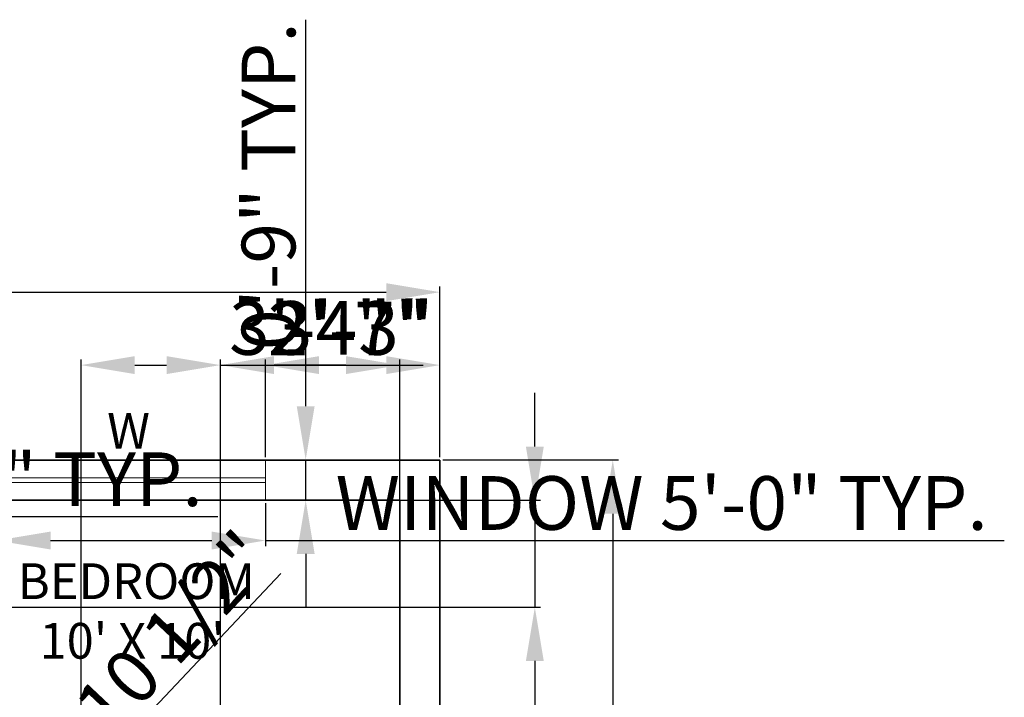
# Model space of a CAD drawing. Units: inches. Extents: x 2122 to 2726, y 1923 to 2370.
# Tile 6 of 6: x 2506 to 2726, y 2218 to 2370. Entities that reach past the tile are written whole.
import ezdxf

# ---------------------------------------------------------------- set-up
doc = ezdxf.new("R2010")
doc.units = ezdxf.units.IN
for name, color, linetype, lineweight in [('A-ANNO-DIMS', 2, 'Continuous', 18), ('A-ANNO-TEXT', 7, 'Continuous', 18), ('A-AREA-IDEN', 7, 'Continuous', 25), ('A-GLAZ', 4, 'Continuous', 18), ('A-WALL', 7, 'Continuous', 35)]:
    doc.layers.add(name, color=color, linetype=linetype, lineweight=lineweight)
doc.styles.get("Standard").update_dxf_attribs({"font": 'arial.ttf'})
doc.dimstyles.new('ISO-25', dxfattribs={"dimtxt": 12, "dimasz": 12, "dimexe": 1.25, "dimexo": 0.625, "dimtad": 1, "dimlunit": 3, "dimtxsty": 'Standard', "dimcen": 2.5, "dimadec": 0, "dimazin": 0, "dimtfac": 1, "dimtmove": 0, "dimatfit": 3, "dimfxl": 1, "dimarcsym": 0})

# ---------------------------------------------------------------- blocks, each defined once
blk = doc.blocks.new('*D9')
at = {"layer": 'A-ANNO-DIMS', "color": 0, "lineweight": -2, "transparency": 16777216}
for p, q in [((2600.63, 2271.24), (2639.88, 2271.24)), ((2638.63, 2259.24), (2638.63, 1984.74)), ((2600.63, 1972.74), (2639.88, 1972.74))]:
    blk.add_line(p, q, dxfattribs=at)
at = {"layer": 'A-ANNO-DIMS', "color": 0, "transparency": 16777216}
for points in [[(2636.63, 2259.24), (2640.63, 2259.24), (2638.63, 2271.24)], [(2636.63, 1984.74), (2640.63, 1984.74), (2638.63, 1972.74)]]:
    blk.add_solid(points, dxfattribs=at)
at = {"layer": 'Defpoints', "color": 0, "transparency": 16777216}
for p in [(2600.01, 2271.24), (2600.01, 1972.74), (2638.63, 1972.74)]:
    blk.add_point(p, dxfattribs=at)
at = {"layer": 'A-ANNO-DIMS', "color": 0, "transparency": 16777216, "insert": (2631.88, 2121.99), "char_height": 12, "attachment_point": 5, "rotation": 90}
blk.add_mtext("25'", dxfattribs=at)
blk = doc.blocks.new('*D10')
at = {"layer": 'A-ANNO-DIMS', "color": 0, "lineweight": -2, "transparency": 16777216}
for p, q in [((2232.51, 2271.86), (2232.51, 2309.99)), ((2244.51, 2308.74), (2588.01, 2308.74)), ((2600.01, 2271.86), (2600.01, 2309.99))]:
    blk.add_line(p, q, dxfattribs=at)
at = {"layer": 'A-ANNO-DIMS', "color": 0, "transparency": 16777216}
for points in [[(2244.51, 2310.74), (2244.51, 2306.74), (2232.51, 2308.74)], [(2588.01, 2310.74), (2588.01, 2306.74), (2600.01, 2308.74)]]:
    blk.add_solid(points, dxfattribs=at)
at = {"layer": 'Defpoints', "color": 0, "transparency": 16777216}
for p in [(2600.01, 2308.74), (2232.51, 2271.24), (2600.01, 2271.24)]:
    blk.add_point(p, dxfattribs=at)
at = {"layer": 'A-ANNO-DIMS', "color": 0, "transparency": 16777216, "insert": (2416.26, 2315.49), "char_height": 12, "attachment_point": 5}
blk.add_mtext("31'", dxfattribs=at)
blk = doc.blocks.new('WIN-60IN')
for p, q in [((0, 0), (0, 9)), ((60, 0), (60, 9)), ((0, 5), (60, 5)), ((0, 4), (60, 4))]:
    blk.add_line(p, q)
blk = doc.blocks.new('*D16')
at = {"layer": 'A-ANNO-DIMS', "color": 0, "lineweight": -2, "transparency": 16777216}
for p, q in [((2501.01, 2261.61), (2501.01, 2251.99)), ((2561.01, 2261.61), (2561.01, 2251.99)), ((2513.01, 2253.24), (2549.01, 2253.24)), ((2561.01, 2253.24), (2726.11, 2253.24))]:
    blk.add_line(p, q, dxfattribs=at)
at = {"layer": 'A-ANNO-DIMS', "color": 0, "transparency": 16777216}
for points in [[(2513.01, 2255.24), (2513.01, 2251.24), (2501.01, 2253.24)], [(2549.01, 2255.24), (2549.01, 2251.24), (2561.01, 2253.24)]]:
    blk.add_solid(points, dxfattribs=at)
at = {"layer": 'Defpoints', "color": 0, "transparency": 16777216}
for p in [(2501.01, 2262.24), (2561.01, 2262.24), (2561.01, 2253.24)]:
    blk.add_point(p, dxfattribs=at)
at = {"layer": 'A-ANNO-DIMS', "color": 0, "transparency": 16777216, "insert": (2649.56, 2260.07), "char_height": 12, "attachment_point": 5}
blk.add_mtext('WINDOW 5\'-0" TYP.', dxfattribs=at)
blk = doc.blocks.new('*D17')
at = {"layer": 'A-ANNO-DIMS', "color": 0, "lineweight": -2, "transparency": 16777216}
for p, q in [((2570.01, 2283.24), (2570.01, 2369.63)), ((2561.63, 2271.24), (2571.26, 2271.24)), ((2570.01, 2262.24), (2570.01, 2271.24)), ((2561.63, 2262.24), (2571.26, 2262.24)), ((2570.01, 2250.24), (2570.01, 2238.24))]:
    blk.add_line(p, q, dxfattribs=at)
at = {"layer": 'A-ANNO-DIMS', "color": 0, "transparency": 16777216}
for points in [[(2568.01, 2283.24), (2572.01, 2283.24), (2570.01, 2271.24)], [(2568.01, 2250.24), (2572.01, 2250.24), (2570.01, 2262.24)]]:
    blk.add_solid(points, dxfattribs=at)
at = {"layer": 'Defpoints', "color": 0, "transparency": 16777216}
for p in [(2561.01, 2271.24), (2570.01, 2271.24), (2561.01, 2262.24)]:
    blk.add_point(p, dxfattribs=at)
at = {"layer": 'A-ANNO-DIMS', "color": 0, "transparency": 16777216, "insert": (2563.26, 2332.43), "char_height": 12, "attachment_point": 5, "rotation": 90}
blk.add_mtext('0\'-9" TYP.', dxfattribs=at)
blk = doc.blocks.new('*D20')
at = {"layer": 'A-ANNO-DIMS', "color": 0, "lineweight": -2, "transparency": 16777216}
for p, q in [((2378.01, 2261.61), (2378.01, 2257.39)), ((2402.01, 2261.61), (2402.01, 2257.39)), ((2366.01, 2258.64), (2354.01, 2258.64)), ((2378.01, 2258.64), (2402.01, 2258.64)), ((2414.01, 2258.64), (2550.39, 2258.64))]:
    blk.add_line(p, q, dxfattribs=at)
at = {"layer": 'A-ANNO-DIMS', "color": 0, "transparency": 16777216}
for points in [[(2366.01, 2260.64), (2366.01, 2256.64), (2378.01, 2258.64)], [(2414.01, 2260.64), (2414.01, 2256.64), (2402.01, 2258.64)]]:
    blk.add_solid(points, dxfattribs=at)
at = {"layer": 'Defpoints', "color": 0, "transparency": 16777216}
for p in [(2378.01, 2262.24), (2402.01, 2262.24), (2402.01, 2258.64)]:
    blk.add_point(p, dxfattribs=at)
at = {"layer": 'A-ANNO-DIMS', "color": 0, "transparency": 16777216, "insert": (2488.2, 2265.39), "char_height": 12, "attachment_point": 5}
blk.add_mtext('VENT 2\'-0" TYP.', dxfattribs=at)
blk = doc.blocks.new('*D42')
at = {"layer": 'A-ANNO-DIMS', "color": 0, "lineweight": -2, "transparency": 16777216}
for p, q in [((2561.01, 2271.86), (2561.01, 2293.69)), ((2573.01, 2292.44), (2588.01, 2292.44)), ((2600.01, 2271.86), (2600.01, 2293.69))]:
    blk.add_line(p, q, dxfattribs=at)
at = {"layer": 'A-ANNO-DIMS', "color": 0, "transparency": 16777216}
for points in [[(2573.01, 2294.44), (2573.01, 2290.44), (2561.01, 2292.44)], [(2588.01, 2294.44), (2588.01, 2290.44), (2600.01, 2292.44)]]:
    blk.add_solid(points, dxfattribs=at)
at = {"layer": 'Defpoints', "color": 0, "transparency": 16777216}
for p in [(2600.01, 2292.44), (2561.01, 2271.24), (2600.01, 2271.24)]:
    blk.add_point(p, dxfattribs=at)
at = {"layer": 'A-ANNO-DIMS', "color": 0, "transparency": 16777216, "insert": (2580.51, 2299.19), "char_height": 12, "attachment_point": 5}
blk.add_mtext('3\'-3"', dxfattribs=at)
blk = doc.blocks.new('*D48')
at = {"layer": 'A-ANNO-DIMS', "color": 0, "lineweight": -2, "transparency": 16777216}
for p, q in [((2519.81, 2071.41), (2519.81, 2293.69)), ((2531.81, 2292.44), (2538.94, 2292.44)), ((2550.94, 2071.41), (2550.94, 2293.69)), ((2550.94, 2292.44), (2596.29, 2292.44))]:
    blk.add_line(p, q, dxfattribs=at)
at = {"layer": 'A-ANNO-DIMS', "color": 0, "transparency": 16777216}
for points in [[(2531.81, 2294.44), (2531.81, 2290.44), (2519.81, 2292.44)], [(2538.94, 2294.44), (2538.94, 2290.44), (2550.94, 2292.44)]]:
    blk.add_solid(points, dxfattribs=at)
at = {"layer": 'Defpoints', "color": 0, "transparency": 16777216}
for p in [(2550.94, 2292.44), (2519.81, 2070.79), (2550.94, 2070.79)]:
    blk.add_point(p, dxfattribs=at)
at = {"layer": 'A-ANNO-DIMS', "color": 0, "transparency": 16777216, "insert": (2579.61, 2299.09), "char_height": 12, "attachment_point": 5}
blk.add_mtext('2\'-7"', dxfattribs=at)
blk = doc.blocks.new('*D57')
at = {"layer": 'A-ANNO-DIMS', "color": 0, "lineweight": -2, "transparency": 16777216}
for p, q in [((2550.94, 2071.41), (2550.94, 2293.69)), ((2579.01, 2292.44), (2562.94, 2292.44)), ((2591.01, 2090.36), (2591.01, 2293.69))]:
    blk.add_line(p, q, dxfattribs=at)
at = {"layer": 'A-ANNO-DIMS', "color": 0, "transparency": 16777216}
for points in [[(2562.94, 2294.44), (2562.94, 2290.44), (2550.94, 2292.44)], [(2579.01, 2294.44), (2579.01, 2290.44), (2591.01, 2292.44)]]:
    blk.add_solid(points, dxfattribs=at)
at = {"layer": 'Defpoints', "color": 0, "transparency": 16777216}
for p in [(2550.94, 2292.44), (2591.01, 2089.74), (2550.94, 2070.79)]:
    blk.add_point(p, dxfattribs=at)
at = {"layer": 'A-ANNO-DIMS', "color": 0, "transparency": 16777216, "insert": (2570.97, 2299.19), "char_height": 12, "attachment_point": 5}
blk.add_mtext('3\'-4"', dxfattribs=at)
blk = doc.blocks.new('*D67')
at = {"layer": 'A-ANNO-DIMS', "color": 0, "lineweight": -2, "transparency": 16777216}
for p, q in [((2621.21, 2274.24), (2621.21, 2286.24)), ((2467.13, 2262.24), (2622.46, 2262.24)), ((2621.21, 2262.24), (2621.21, 2238.32)), ((2461.84, 2238.32), (2622.46, 2238.32)), ((2621.21, 2226.32), (2621.21, 2180.97))]:
    blk.add_line(p, q, dxfattribs=at)
at = {"layer": 'A-ANNO-DIMS', "color": 0, "transparency": 16777216}
for points in [[(2619.21, 2274.24), (2623.21, 2274.24), (2621.21, 2262.24)], [(2619.21, 2226.32), (2623.21, 2226.32), (2621.21, 2238.32)]]:
    blk.add_solid(points, dxfattribs=at)
at = {"layer": 'Defpoints', "color": 0, "transparency": 16777216}
for p in [(2466.51, 2262.24), (2461.22, 2238.32), (2621.21, 2238.32)]:
    blk.add_point(p, dxfattribs=at)
at = {"layer": 'A-ANNO-DIMS', "color": 0, "transparency": 16777216, "insert": (2614.46, 2197.64), "char_height": 12, "attachment_point": 5, "rotation": 90}
blk.add_mtext('2\'-0"', dxfattribs=at)
blk = doc.blocks.new('*D71')
at = {"layer": 'A-ANNO-DIMS', "color": 0, "lineweight": -2, "transparency": 16777216}
for p, q in [((2564.44, 2245.87), (2499.95, 2177.59)), ((2468.06, 2143.82), (2491.71, 2168.87))]:
    blk.add_line(p, q, dxfattribs=at)
at = {"layer": 'A-ANNO-DIMS', "color": 0, "transparency": 16777216}
blk.add_solid([(2498.5, 2178.96), (2501.41, 2176.22), (2491.71, 2168.87)], dxfattribs=at)
at = {"layer": 'Defpoints', "color": 0, "transparency": 16777216}
for p in [(2491.71, 2168.87), (2468.06, 2143.82)]:
    blk.add_point(p, dxfattribs=at)
at = {"layer": 'A-ANNO-DIMS', "color": 0, "transparency": 16777216, "insert": (2531.35, 2220.78), "char_height": 12, "attachment_point": 5, "rotation": 46.6362}
blk.add_mtext('R2\'-10 1/2"', dxfattribs=at)

msp = doc.modelspace()

# ---------------------------------------------------------------- linework, layer by layer
at = {"layer": 'A-WALL'}
for p, q in [((2232.508, 2271.236), (2600.008, 2271.236)), ((2600.008, 1972.736), (2600.008, 2271.236)), ((2471.008, 2262.236), (2591.008, 2262.236)), ((2591.008, 2142.236), (2591.008, 2262.236))]:
    msp.add_line(p, q, dxfattribs=at)

# ---------------------------------------------------------------- block references
at = {"layer": 'A-GLAZ'}
msp.add_blockref('WIN-60IN', (2501.008, 2262.236), dxfattribs=at)

# ---------------------------------------------------------------- texts
at = {"layer": 'A-ANNO-TEXT', "insert": (2525.642, 2281.742), "char_height": 7.99, "attachment_point": 1}
msp.add_mtext_dynamic_manual_height_columns('W', width=65.06795, gutter_width=39.949, heights=[0], dxfattribs=at)
at = {"layer": 'A-AREA-IDEN', "insert": (2505.67, 2248.148), "char_height": 7.98971, "attachment_point": 1}
msp.add_mtext_dynamic_manual_height_columns("BEDROOM \\P  10' X 10'", width=65.06795, gutter_width=39.949, heights=[0], dxfattribs=at)

# ---------------------------------------------------------------- dimensions: what is measured, and where the dimension line sits
at = {"layer": 'A-ANNO-DIMS'}
for base, p1, p2, text, override, picture, middle in [((2570.008, 2271.236), (2561.008, 2262.236), (2561.008, 2271.236), '<> TYP.', {"dimdec": 1, "dimlfac": 1, "dimrnd": 0, "dimzin": 1, "dimdsep": 46, "dimlunit": 4, "dimfrac": 2}, '*D17', (2563.256, 2332.434)), ((2638.632, 1972.736), (2600.008, 2271.236), (2600.008, 1972.736), "25'", {"dimclrd": 0, "dimclre": 0, "dimclrt": 0}, '*D9', (2631.88, 2121.986))]:
    dim = msp.add_linear_dim(base=base, p1=p1, p2=p2, angle=90, text=text, dimstyle='ISO-25', override=override, dxfattribs=at)
    dim.commit()
    dim.dimension.update_dxf_attribs({"geometry": picture, "text_midpoint": middle})
for base, p1, p2, text, override, picture, middle in [((2600.008, 2308.735), (2232.508, 2271.236), (2600.008, 2271.236), "31'", {"dimclrd": 0, "dimclre": 0, "dimclrt": 0}, '*D10', (2416.258, 2315.491)), ((2402.008, 2258.636), (2378.008, 2262.236), (2402.008, 2262.236), 'VENT <> TYP.', {"dimdec": 1, "dimlfac": 1, "dimrnd": 0, "dimzin": 1, "dimdsep": 46, "dimlunit": 4, "dimfrac": 2}, '*D20', (2488.2, 2265.388)), ((2561.008, 2253.236), (2501.008, 2262.236), (2561.008, 2262.236), 'WINDOW <> TYP.', {"dimdec": 1, "dimlfac": 1, "dimrnd": 0, "dimzin": 1, "dimdsep": 46, "dimlunit": 4, "dimfrac": 2}, '*D16', (2649.558, 2260.07))]:
    dim = msp.add_linear_dim(base=base, p1=p1, p2=p2, text=text, dimstyle='ISO-25', override=override, dxfattribs=at)
    dim.commit()
    dim.dimension.update_dxf_attribs({"geometry": picture, "text_midpoint": middle})
for base, p1, p2, picture, middle in [((2550.937, 2292.436), (2519.809, 2070.789), (2550.937, 2070.789), '*D48', (2579.614, 2299.086)), ((2550.937, 2292.436), (2591.008, 2089.736), (2550.937, 2070.789), '*D57', (2570.973, 2299.192)), ((2600.008, 2292.436), (2561.008, 2271.236), (2600.008, 2271.236), '*D42', (2580.508, 2299.192))]:
    dim = msp.add_linear_dim(base=base, p1=p1, p2=p2, dimstyle='ISO-25', override={"dimdec": 1, "dimlfac": 1, "dimrnd": 0, "dimzin": 1, "dimdsep": 46, "dimlunit": 4, "dimfrac": 2}, dxfattribs=at)
    dim.commit()
    dim.dimension.update_dxf_attribs({"geometry": picture, "text_midpoint": middle})
dim = msp.add_linear_dim(base=(2621.208, 2238.321), p1=(2466.508, 2262.236), p2=(2461.216, 2238.321), angle=90, dimstyle='ISO-25', override={"dimdec": 1, "dimlfac": 1, "dimrnd": 0, "dimzin": 1, "dimdsep": 46, "dimlunit": 4, "dimfrac": 2}, dxfattribs=at)
dim.commit()
dim.dimension.update_dxf_attribs({"geometry": '*D67', "text_midpoint": (2614.456, 2197.644)})
dim = msp.add_radius_dim(center=(2468.058, 2143.819), mpoint=(2491.714, 2168.866), dimstyle='ISO-25', override={"dimdec": 1, "dimlfac": 1, "dimrnd": 0, "dimzin": 1, "dimdsep": 46, "dimlunit": 4, "dimfrac": 2}, dxfattribs=at)
dim.commit()
dim.dimension.update_dxf_attribs({"geometry": '*D71', "text_midpoint": (2531.352, 2220.781)})

doc.saveas('drawing.dxf')
